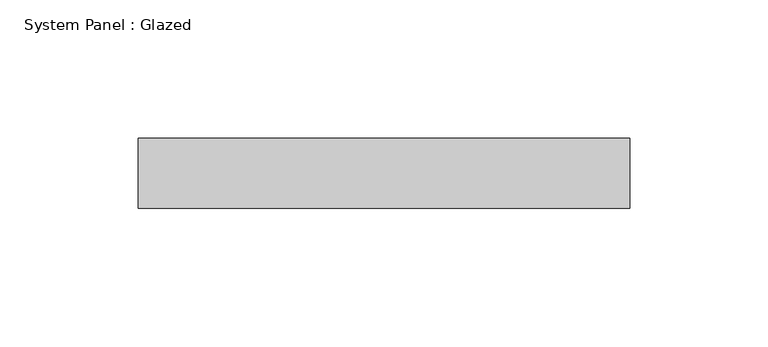
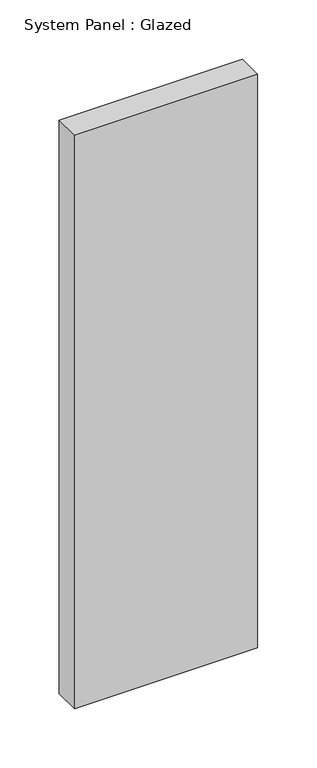
"""IFC4 building model written with IfcOpenShell, lengths in millimetres: plate geometry, System Panel : Glazed."""

from ifc_helpers import new_model, si_unit, origin, origin_with_axes, place, context, project, spatial, polyline, outline, extrude, source, transform, mapped, element, save


def system_panel_glazed_c39d0069(model_context):
    return source(origin(), model_context, "Body", "SweptSolid", [
        extrude(outline(polyline([(88.9, 19.05), (-88.9, 19.05), (-88.9, 44.45), (88.9, 44.45), (88.9, 19.05)])), origin_with_axes(), (0.0, 0.0, 1.0), 588.5125925),
    ])


if __name__ == "__main__":
    model = new_model("IFC4")
    model_context = context("Model", 3, world=origin())
    ifc_project = project(units=[si_unit("LENGTHUNIT", "METRE", prefix="MILLI")], contexts=[model_context])
    site = spatial("IfcSite", under=ifc_project)
    building = spatial("IfcBuilding", under=site)
    placement = place(None, origin())
    system_panel_glazed_shape = system_panel_glazed_c39d0069(model_context)
    element("IfcPlate", 1, ObjectType="System Panel : Glazed", at=placement, inside=building, context=model_context, shape_type="MappedRepresentation", body=[
        mapped(system_panel_glazed_shape, transform((0.0, 0.0, 0.0), x_axis=(1.0, 0.0, 0.0), y_axis=(0.0, 1.0, 0.0), z_axis=(0.0, 0.0, 1.0))),
    ])
    save(model, "model.ifc")

# Revit data of these elements
# Type "System Panel : Glazed"
#   Construction Type Id = "GSP4R"
#   Analytic Construction = "1/8 in Pilkington single glazing"
#   Visual Light Transmittance = 0.9
#   Solar Heat Gain Coefficient = 0.86
#   Heat Transfer Coefficient (U) = 1.18115 BTU/(h·ft²·°F)
#   Define Thermal Properties by = 1
# Element 1 (IfcPlate, "System Panel : Glazed")
#   Materials on its faces: "Glass"
# Materials
#   "Glass": class "Glass", colour RGB 0 128 192, transparency 0.75, Description = "Soda Lime Glass", Cost = 0
